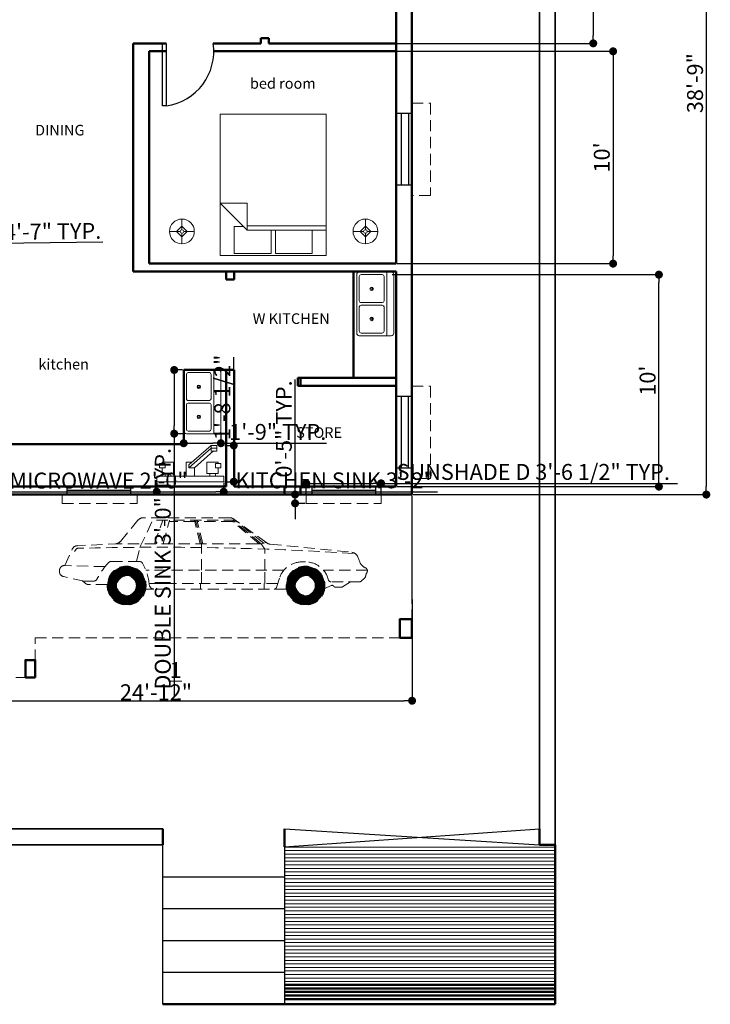
# Model space of a CAD drawing. Units: inches. Extents: x 2050 to 6806, y 2092 to 5743.
# Tile 2 of 8: x 2600 to 2991, y 2149 to 2706. Entities that reach past the tile are written whole.
import ezdxf

# ---------------------------------------------------------------- set-up
doc = ezdxf.new("R2010")
doc.units = ezdxf.units.IN
doc.linetypes.add('HIDDEN', pattern=[9.525, 6.35, -3.175])
for name, color, linetype, lineweight in [('A-ANNO-DIMS', 2, 'Continuous', 18), ('A-AREA-IDEN', 7, 'Continuous', 18), ('A-DOOR', 2, 'Continuous', 25), ('A-FLOR-FIXT', 4, 'Continuous', 18), ('A-FLOR-OVHD', 30, 'HIDDEN', 18), ('A-FLOR-PATT', 8, 'Continuous', 13), ('A-FLOR-STRS', 3, 'Continuous', 25), ('A-FURN', 5, 'Continuous', 18), ('A-GLAZ', 6, 'Continuous', 25), ('A-WALL', 7, 'Continuous', 50), ('C-PROP', 90, 'Continuous', 35)]:
    doc.layers.add(name, color=color, linetype=linetype, lineweight=lineweight)
doc.styles.get("Standard").update_dxf_attribs({"font": 'arial.ttf'})
doc.dimstyles.new('ISO-25', dxfattribs={"dimtxt": 9, "dimasz": 4.5, "dimexe": 1.25, "dimexo": 0.625, "dimtad": 1, "dimdec": 1, "dimlunit": 4, "dimtxsty": 'Standard', "dimblk": 'DOT', "dimcen": 2.5, "dimadec": 0, "dimazin": 0, "dimtfac": 1, "dimtdec": 1, "dimtmove": 0, "dimatfit": 3, "dimldrblk": 'ARCHTICK', "dimfxl": 1, "dimarcsym": 0})

# ---------------------------------------------------------------- blocks, each defined once
blk = doc.blocks.new('Faucet - kit sink front')
for p, q in [((-0.25, 3), (3.75, 6.5)), ((3.75, 6), (-0.25, 2.5)), ((4.1921, 5.5041), (0.75, 2.5)), ((3.75, 6), (3.75, 6.5)), ((3.75, 6.5), (4.75, 6.5)), ((3.75, 5.5), (3.75, 6)), ((4.75, 6), (3.75, 6)), ((4.75, 5.5), (3.75, 5.5)), ((4.75, 6.5), (4.75, 6)), ((4.75, 6), (4.75, 5.5)), ((-0.75, 3.5), (0.3192, 3.5)), ((-0.75, 1), (-0.75, 3.5)), ((-0.25, 2.5), (-0.25, 3)), ((0.75, 2.5), (-0.25, 2.5)), ((0.75, 2.5), (0.75, 1)), ((-4.5, 1), (-4.5, 1.5)), ((-3.5, 1.5), (-3.5, 1)), ((3.5, 1.5), (3.5, 1)), ((4.5, 1), (4.5, 1.5))]:
    blk.add_line(p, q)
for points in [[(-5.5, 2.5), (-5.5, 3.25), (-4.5, 3.25), (-4.5, 2.5)], [(5.5, 2.5), (5.5, 3.25), (4.5, 3.25), (4.5, 2.5)], [(-6, 0), (-6, 1), (6, 1), (6, 0)]]:
    blk.add_lwpolyline(points, close=True)
for points in [[(-5, 3.2513), (-5, 3.5), (-3, 3.5), (-3, 1.5), (-5, 1.5), (-5, 2.5)], [(5, 3.2513), (5, 3.5), (3, 3.5), (3, 1.5), (5, 1.5), (5, 2.5)]]:
    blk.add_lwpolyline(points)
blk = doc.blocks.new('Sink-double - 36 in top')
for p, q in [((-18, -4), (18, -4)), ((-0.75, -18.5), (-0.75, -6.5)), ((0.75, -6.5), (0.75, -18.5))]:
    blk.add_line(p, q)
for points in [[(-16.5, 0), (16.5, 0)], [(-18, -19.5), (-18, -1.5)], [(-15.5, -5.5), (-1.75, -5.5)], [(1.75, -5.5), (15.5, -5.5)], [(18, -1.5), (18, -19.5)], [(-16.5, -18.5), (-16.5, -6.5)], [(16.5, -6.5), (16.5, -18.5)], [(16.5, -21), (-16.5, -21)], [(-1.75, -19.5), (-15.5, -19.5)], [(15.5, -19.5), (1.75, -19.5)]]:
    blk.add_lwpolyline(points)
for centre, radius in [((-8.5, -12.5), 1), ((-8.5, -12.5), 0.5), ((8.5, -12.5), 1), ((8.5, -12.5), 0.5)]:
    blk.add_circle(centre, radius)
for centre, radius, start, end in [((-16.5, -1.5), 1.5, 90, 180), ((16.5, -1.5), 1.5, 0, 90), ((-15.5, -6.5), 1, 90, 180), ((-1.75, -6.5), 1, 0, 90), ((1.75, -6.5), 1, 90, 180), ((15.5, -6.5), 1, 0, 90), ((-16.5, -19.5), 1.5, 180, 270), ((-15.5, -18.5), 1, 180, 270), ((-1.75, -18.5), 1, 270, 0), ((1.75, -18.5), 1, 180, 270), ((15.5, -18.5), 1, 270, 0), ((16.5, -19.5), 1.5, 270, 0)]:
    blk.add_arc(centre, radius, start, end)
blk = doc.blocks.new('Bed - Queen')
for p, q in [((0, -80.00003), (0, 0)), ((0, 0), (59.99999, 0)), ((59.99999, 0), (59.99999, -80.00003)), ((7.99999, -1.2), (28.79998, -1.2)), ((7.99999, -14.4), (7.99999, -1.2)), ((28.79998, -1.2), (28.79998, -14.4)), ((31.19999, -1.2), (51.99999, -1.2)), ((31.19999, -14.4), (31.19999, -1.2)), ((51.99999, -1.2), (51.99999, -16.4)), ((0, -14.4), (44.8, -14.4)), ((59.99999, -29.6), (44.8, -14.4)), ((44.8, -14.4), (44.8, -29.6)), ((51.99999, -16.4), (46.79936, -16.4)), ((44.8, -16.8), (0, -16.8)), ((44.8, -29.6), (59.99999, -29.6)), ((59.99999, -80.00003), (0, -80.00003))]:
    blk.add_line(p, q)
blk = doc.blocks.new('Lamp - Table')
for p, q in [((0, 7), (0, 1)), ((-1, 0), (-7, 0)), ((0, 3), (-3, 0)), ((-3, 0), (0, -3)), ((3, 0), (0, 3)), ((0, -3), (3, 0)), ((1, 0), (7, 0)), ((0, -1), (0, -7))]:
    blk.add_line(p, q)
for radius in [7, 1]:
    blk.add_circle((0, 0), radius)
blk = doc.blocks.new('Car - sedan  side')
for p, q in [((-139.53, 35.99), (-129.64, 47.91)), ((-128.57, 32.64), (-121.22, 48.02)), ((-77.81, 49.34), (-126.58, 49.34)), ((-74.7, 48.02), (-121.22, 48.02)), ((-120.32, 34.67), (-115.67, 48.02)), ((-115.4, 34.67), (-111.74, 48.02)), ((-97.55, 47.3), (-111.94, 47.3)), ((-94.41, 34.67), (-97.73, 48.02)), ((-93.72, 34.67), (-97.04, 48.02)), ((-93.03, 34.67), (-96.34, 48.02)), ((-76.26, 47.3), (-96.16, 47.3)), ((-61.08, 34.66), (-76.26, 47.3)), ((-60.02, 34.65), (-76.07, 48.02)), ((-56.87, 35.13), (-75.48, 48.59)), ((-58.54, 34.93), (-74.99, 48.02)), ((-140.23, 34.67), (-163.88, 33.56)), ((-62.28, 34.67), (-140.23, 34.67)), ((-93.72, 19.62), (-93.72, 34.67)), ((-62.28, 34.67), (-60.02, 34.65)), ((-60.02, 34.65), (-58.54, 34.93)), ((-57.97, 31.61), (-60.02, 34.65)), ((-57.21, 35.38), (-58.54, 34.93)), ((-54.93, 34.4), (-8.75, 29.8)), ((-170.93, 22.32), (-166.81, 31.56)), ((-164.57, 31.6), (-165.48, 30.35)), ((-130.39, 24.63), (-128.57, 32.64)), ((-57.97, 19.62), (-57.97, 31.61)), ((-148.26, 21.7), (-171.11, 22.33)), ((-128.78, 24.63), (-144.79, 24.63)), ((-36.97, 24.38), (-34.94, 24.38)), ((-4.21, 24.18), (-5.42, 27.27)), ((-174, 19.51), (-174, 18.91)), ((-47.2, 19.62), (-125.23, 19.62)), ((-93.72, 12.14), (-93.72, 19.62)), ((-57.97, 12.14), (-57.97, 19.62)), ((0, 19.62), (-24.7, 19.62)), ((-160.12, 13.48), (-171.81, 16.16)), ((-159.22, 12.14), (-161.08, 13.7)), ((-155.01, 13.48), (-160.12, 13.48)), ((-147.03, 11.6), (-157.73, 11.6)), ((-50.67, 12.14), (-123.32, 12.14)), ((-94.21, 9.03), (-94.21, 12.14)), ((-58.39, 9.03), (-58.39, 12.14)), ((-51.4, 9.89), (-49.69, 15.14)), ((-4.23, 13.19), (-20.72, 13.19)), ((-9.5, 13.19), (-14.1, 10.2)), ((-3.22, 13.59), (-1.77, 14.97)), ((-120.62, 9.03), (-125.23, 9.03)), ((-45.76, 9.03), (-120.62, 9.03)), ((-20.36, 11.06), (-24.06, 9.44)), ((-18.83, 10.42), (-19.11, 10.76)), ((-14.68, 10.03), (-18.01, 10.03))]:
    blk.add_line(p, q)
at = {"const_width": 5.49}
for points in [[(-127.8, 11, -1), (-144.3, 11, -1)], [(-26.69, 11, -1), (-43.19, 11, -1)]]:
    blk.add_lwpolyline(points, format="xyb", close=True, dxfattribs=at)
for centre, radius in [((-136.05, 11), 11), ((-34.94, 11), 11), ((-136.05, 11), 5.51), ((-34.94, 11), 5.51)]:
    blk.add_circle(centre, radius)
for centre, radius, start, end in [((-126.58, 45.38), 3.97, 90, 140.3029), ((-77.81, 45.38), 3.97, 54.135, 90), ((-163.72, 30.18), 3.38, 92.6827, 155.9736), ((-142.58, 38.53), 3.97, 272.6827, 320.3029), ((-54.54, 38.35), 3.97, 234.135, 264.3123), ((-163.62, 30.91), 1.17, 91.491, 143.9553), ((-118.51, -1702.12), 1734.79, 86.34698, 91.49105), ((-9.15, 25.82), 4, 21.3107, 84.3123), ((-171.18, 19.51), 2.82, 88.4193, 180), ((-118.09, -2.78), 38.85, 136.3964, 152.9097), ((-144.79, 22.64), 1.98, 90, 136.3964), ((-128.78, 22.64), 1.98, 28.1371, 90), ((-157.14, 7.48), 34.14, 6.5135, 28.1371), ((-36.97, 11), 13.38, 90, 161.9732), ((-34.94, 11), 13.38, 13.5864, 90), ((0.9, 26.18), 5.49, 201.3107, 247.7048), ((-171.18, 18.91), 2.82, 180, 257.0905), ((-3.82, 17.12), 2.96, 313.7173, 352.3839), ((-1.92, 19.3), 1.94, 325.3744, 67.7048), ((2.46, 16.28), 3.37, 145.3744, 172.3839), ((-157.73, 13.93), 2.32, 230.1291, 270), ((-155.01, 16.1), 2.62, 270, 332.9097), ((-120.62, 11.65), 2.62, 186.5135, 270), ((-20.72, 14.43), 1.24, 193.5864, 270), ((-19.93, 10.09), 1.06, 39.301, 113.7159), ((-4.23, 14.65), 1.46, 270, 313.7173), ((-52.58, 10.27), 1.24, 270, 341.9732), ((-18.01, 11.09), 1.06, 219.301, 270), ((-14.68, 11.09), 1.06, 270, 303.047)]:
    blk.add_arc(centre, radius, start, end)
blk = doc.blocks.new('_Dot')
at = {"color": 0, "linetype": 'ByBlock', "lineweight": -2}
blk.add_line((-0.5, 0), (-1, 0), dxfattribs=at)
at = {"color": 0, "linetype": 'ByBlock', "const_width": 0.5}
blk.add_lwpolyline([(-0.25, 0, 1), (0.25, 0, 1)], format="xyb", close=True, dxfattribs=at)
blk = doc.blocks.new('*D32')
at = {"layer": 'A-ANNO-DIMS', "color": 0, "lineweight": -2, "transparency": 16777216}
for p, q in [((2532.41, 2436.47), (2532.47, 2319.32)), ((2821.91, 2436.61), (2821.97, 2319.47)), ((2536.97, 2320.57), (2817.47, 2320.71))]:
    blk.add_line(p, q, dxfattribs=at)
at = {"layer": 'Defpoints', "color": 0, "transparency": 16777216}
for p in [(2821.91, 2437.24), (2532.41, 2437.09), (2821.97, 2320.72)]:
    blk.add_point(p, dxfattribs=at)
at = {"layer": 'A-ANNO-DIMS', "color": 0, "lineweight": -2, "transparency": 16777216, "xscale": 4.5, "yscale": 4.5, "zscale": 4.5}
for p, rotation in [((2532.47, 2320.57), 180.0291193537901), ((2821.97, 2320.72), 0.029119353790171)]:
    blk.add_blockref('_Dot', p, dxfattribs=dict(at, rotation=rotation))
at = {"layer": 'A-ANNO-DIMS', "color": 0, "transparency": 16777216, "insert": (2677.21, 2331.81), "char_height": 9, "attachment_point": 5, "rotation": 0.0291}
blk.add_mtext('24\'-1{\\H1x;\\S1/2;}"', dxfattribs=at)
blk = doc.blocks.new('_ArchTick')
at = {"color": 0, "linetype": 'ByBlock', "const_width": 0.15}
blk.add_lwpolyline([(-0.5, -0.5), (0.5, 0.5)], dxfattribs=at)
blk = doc.blocks.new('*D33')
at = {"layer": 'A-ANNO-DIMS', "color": 0, "lineweight": -2, "transparency": 16777216}
for p, q in [((2810.78, 2561.51), (2962.71, 2561.51)), ((2961.46, 2446.24), (2961.46, 2557.01)), ((2813.53, 2441.74), (2962.71, 2441.74))]:
    blk.add_line(p, q, dxfattribs=at)
at = {"layer": 'Defpoints', "color": 0, "transparency": 16777216}
for p in [(2810.15, 2561.51), (2961.46, 2561.51), (2812.91, 2441.74)]:
    blk.add_point(p, dxfattribs=at)
at = {"layer": 'A-ANNO-DIMS', "color": 0, "lineweight": -2, "transparency": 16777216, "xscale": 4.5, "yscale": 4.5, "zscale": 4.5}
for p, rotation in [((2961.46, 2561.51), 90), ((2961.46, 2441.74), 270)]:
    blk.add_blockref('_Dot', p, dxfattribs=dict(at, rotation=rotation))
at = {"layer": 'A-ANNO-DIMS', "color": 0, "transparency": 16777216, "insert": (2956.24, 2501.62), "char_height": 9, "attachment_point": 5, "rotation": 90}
blk.add_mtext("10'", dxfattribs=at)
blk = doc.blocks.new('*D34')
at = {"layer": 'A-ANNO-DIMS', "color": 0, "lineweight": -2, "transparency": 16777216}
for p, q in [((2822.53, 2902.24), (2989.52, 2902.24)), ((2988.27, 2897.74), (2988.27, 2441.74)), ((2822.53, 2437.24), (2989.52, 2437.24))]:
    blk.add_line(p, q, dxfattribs=at)
at = {"layer": 'Defpoints', "color": 0, "transparency": 16777216}
for p in [(2821.91, 2902.24), (2821.91, 2437.24), (2988.27, 2437.24)]:
    blk.add_point(p, dxfattribs=at)
at = {"layer": 'A-ANNO-DIMS', "color": 0, "lineweight": -2, "transparency": 16777216, "xscale": 4.5, "yscale": 4.5, "zscale": 4.5}
for p, rotation in [((2988.27, 2902.24), 90), ((2988.27, 2437.24), 270)]:
    blk.add_blockref('_Dot', p, dxfattribs=dict(at, rotation=rotation))
at = {"layer": 'A-ANNO-DIMS', "color": 0, "transparency": 16777216, "insert": (2983.05, 2669.74), "char_height": 9, "attachment_point": 5, "rotation": 90}
blk.add_mtext('38\'-9"', dxfattribs=at)
blk = doc.blocks.new('*D35')
at = {"layer": 'A-ANNO-DIMS', "color": 0, "lineweight": -2, "transparency": 16777216}
for p, q in [((2813.53, 2687.74), (2936.83, 2687.74)), ((2935.58, 2683.24), (2935.58, 2572.24)), ((2813.53, 2567.74), (2936.83, 2567.74))]:
    blk.add_line(p, q, dxfattribs=at)
at = {"layer": 'Defpoints', "color": 0, "transparency": 16777216}
for p in [(2812.91, 2687.74), (2812.91, 2567.74), (2935.58, 2567.74)]:
    blk.add_point(p, dxfattribs=at)
at = {"layer": 'A-ANNO-DIMS', "color": 0, "lineweight": -2, "transparency": 16777216, "xscale": 4.5, "yscale": 4.5, "zscale": 4.5}
for p, rotation in [((2935.58, 2687.74), 90), ((2935.58, 2567.74), 270)]:
    blk.add_blockref('_Dot', p, dxfattribs=dict(at, rotation=rotation))
at = {"layer": 'A-ANNO-DIMS', "color": 0, "transparency": 16777216, "insert": (2930.36, 2627.74), "char_height": 9, "attachment_point": 5, "rotation": 90}
blk.add_mtext("10'", dxfattribs=at)
blk = doc.blocks.new('*D36')
at = {"layer": 'A-ANNO-DIMS', "color": 0, "lineweight": -2, "transparency": 16777216}
for p, q in [((2809.63, 2740.24), (2925.62, 2740.24)), ((2924.37, 2735.74), (2924.37, 2696.74)), ((2813.53, 2692.24), (2925.62, 2692.24))]:
    blk.add_line(p, q, dxfattribs=at)
at = {"layer": 'Defpoints', "color": 0, "transparency": 16777216}
for p in [(2809.01, 2740.24), (2812.91, 2692.24), (2924.37, 2692.24)]:
    blk.add_point(p, dxfattribs=at)
at = {"layer": 'A-ANNO-DIMS', "color": 0, "lineweight": -2, "transparency": 16777216, "xscale": 4.5, "yscale": 4.5, "zscale": 4.5}
for p, rotation in [((2924.37, 2740.24), 90), ((2924.37, 2692.24), 270)]:
    blk.add_blockref('_Dot', p, dxfattribs=dict(at, rotation=rotation))
at = {"layer": 'A-ANNO-DIMS', "color": 0, "transparency": 16777216, "insert": (2919.24, 2716.24), "char_height": 9, "attachment_point": 5, "rotation": 90}
blk.add_mtext("4'", dxfattribs=at)
blk = doc.blocks.new('DOOR-750')
blk.add_lwpolyline([(28.97, 0), (26.83, 0), (26.83, 35.38), (28.97, 35.38)], close=True)
blk.add_arc((31.25, 4.42), 31.27, 98.1233, 188.1233)
blk = doc.blocks.new('WIN-1050')
for p, q in [((0, 40.58), (9, 40.58)), ((2.5, 0), (2.5, 40.58)), ((6.5, 0), (6.5, 40.58)), ((0, 0), (9, 0))]:
    blk.add_line(p, q)
blk = doc.blocks.new('SUNSHADE-A')
for p, q in [((0, 52.08), (10.45, 52.08)), ((10.45, 52.08), (10.45, 0)), ((10.45, 0), (0, 0))]:
    blk.add_line(p, q)
blk = doc.blocks.new('SUNSHADE-D')
for p, q in [((0, 4.96), (0, 0)), ((0, 0), (42.28, 0)), ((42.28, 0), (42.28, 4.96))]:
    blk.add_line(p, q)
blk = doc.blocks.new('*D85')
at = {"layer": 'A-ANNO-DIMS', "color": 0, "lineweight": -2, "transparency": 16777216}
for p, q in [((2762.19, 2437.86), (2762.19, 2444.83)), ((2766.69, 2443.58), (2799.97, 2443.58)), ((2804.47, 2437.86), (2804.47, 2444.83)), ((2804.47, 2443.58), (2971.94, 2443.58))]:
    blk.add_line(p, q, dxfattribs=at)
at = {"layer": 'Defpoints', "color": 0, "transparency": 16777216}
for p in [(2804.47, 2443.58), (2762.19, 2437.24), (2804.47, 2437.24)]:
    blk.add_point(p, dxfattribs=at)
at = {"layer": 'A-ANNO-DIMS', "color": 0, "lineweight": -2, "transparency": 16777216, "xscale": 4.5, "yscale": 4.5, "zscale": 4.5, "rotation": 180}
blk.add_blockref('_Dot', (2762.19, 2443.58), dxfattribs=at)
at = {"layer": 'A-ANNO-DIMS', "color": 0, "lineweight": -2, "transparency": 16777216, "xscale": 4.5, "yscale": 4.5, "zscale": 4.5}
blk.add_blockref('_Dot', (2804.47, 2443.58), dxfattribs=at)
at = {"layer": 'A-ANNO-DIMS', "color": 0, "transparency": 16777216, "insert": (2890.45, 2448.86), "char_height": 9, "attachment_point": 5}
blk.add_mtext('SUNSHADE D 3\'-6 1/2" TYP.', dxfattribs=at)
blk = doc.blocks.new('*D86')
at = {"layer": 'A-ANNO-DIMS', "color": 0, "lineweight": -2, "transparency": 16777216}
for p, q in [((2755.85, 2441.74), (2755.85, 2502.35)), ((2761.56, 2437.24), (2754.6, 2437.24)), ((2755.85, 2432.27), (2755.85, 2437.24)), ((2761.56, 2432.27), (2754.6, 2432.27)), ((2755.85, 2427.77), (2755.85, 2423.27))]:
    blk.add_line(p, q, dxfattribs=at)
at = {"layer": 'Defpoints', "color": 0, "transparency": 16777216}
for p in [(2755.85, 2437.24), (2762.19, 2437.24), (2762.19, 2432.27)]:
    blk.add_point(p, dxfattribs=at)
at = {"layer": 'A-ANNO-DIMS', "color": 0, "lineweight": -2, "transparency": 16777216, "xscale": 4.5, "yscale": 4.5, "zscale": 4.5}
for p, rotation in [((2755.85, 2437.24), 270), ((2755.85, 2432.27), 90)]:
    blk.add_blockref('_Dot', p, dxfattribs=dict(at, rotation=rotation))
at = {"layer": 'A-ANNO-DIMS', "color": 0, "transparency": 16777216, "insert": (2750.63, 2474.29), "char_height": 9, "attachment_point": 5, "rotation": 90}
blk.add_mtext('0\'-5" TYP.', dxfattribs=at)
blk = doc.blocks.new('*D91')
at = {"layer": 'A-ANNO-DIMS', "color": 0, "lineweight": -2, "transparency": 16777216}
for p, q in [((2692.28, 2507.65), (2686.26, 2507.65)), ((2687.51, 2503.15), (2687.51, 2476.15)), ((2692.28, 2471.65), (2686.26, 2471.65)), ((2687.51, 2471.65), (2687.51, 2323.46))]:
    blk.add_line(p, q, dxfattribs=at)
at = {"layer": 'Defpoints', "color": 0, "transparency": 16777216}
for p in [(2692.91, 2507.65), (2687.51, 2471.65), (2692.91, 2471.65)]:
    blk.add_point(p, dxfattribs=at)
at = {"layer": 'A-ANNO-DIMS', "color": 0, "lineweight": -2, "transparency": 16777216, "xscale": 4.5, "yscale": 4.5, "zscale": 4.5}
for p, rotation in [((2687.51, 2507.65), 90), ((2687.51, 2471.65), 270)]:
    blk.add_blockref('_Dot', p, dxfattribs=dict(at, rotation=rotation))
at = {"layer": 'A-ANNO-DIMS', "color": 0, "transparency": 16777216, "insert": (2682.22, 2395.31), "char_height": 9, "attachment_point": 5, "rotation": 90}
blk.add_mtext('DOUBLE SINK 3\'-0" TYP.', dxfattribs=at)
blk = doc.blocks.new('*D92')
at = {"layer": 'A-ANNO-DIMS', "color": 0, "lineweight": -2, "transparency": 16777216}
for p, q in [((2692.91, 2471.03), (2692.91, 2465)), ((2713.91, 2471.03), (2713.91, 2465)), ((2697.41, 2466.25), (2709.41, 2466.25)), ((2713.91, 2466.25), (2773.67, 2466.25))]:
    blk.add_line(p, q, dxfattribs=at)
at = {"layer": 'Defpoints', "color": 0, "transparency": 16777216}
for p in [(2692.91, 2471.65), (2713.91, 2471.65), (2713.91, 2466.25)]:
    blk.add_point(p, dxfattribs=at)
at = {"layer": 'A-ANNO-DIMS', "color": 0, "lineweight": -2, "transparency": 16777216, "xscale": 4.5, "yscale": 4.5, "zscale": 4.5, "rotation": 180}
blk.add_blockref('_Dot', (2692.91, 2466.25), dxfattribs=at)
at = {"layer": 'A-ANNO-DIMS', "color": 0, "lineweight": -2, "transparency": 16777216, "xscale": 4.5, "yscale": 4.5, "zscale": 4.5}
blk.add_blockref('_Dot', (2713.91, 2466.25), dxfattribs=at)
at = {"layer": 'A-ANNO-DIMS', "color": 0, "transparency": 16777216, "insert": (2746.04, 2471.47), "char_height": 9, "attachment_point": 5}
blk.add_mtext('1\'-9" TYP.', dxfattribs=at)
blk = doc.blocks.new('*D94')
at = {"layer": 'A-ANNO-DIMS', "color": 0, "lineweight": -2, "transparency": 16777216}
for p, q in [((2530.99, 2591.58), (2531.18, 2577.3)), ((2585.99, 2592.28), (2586.17, 2578.01)), ((2535.66, 2578.61), (2581.66, 2579.2)), ((2586.16, 2579.26), (2647.12, 2580.04))]:
    blk.add_line(p, q, dxfattribs=at)
at = {"layer": 'Defpoints', "color": 0, "transparency": 16777216}
for p in [(2530.98, 2592.2), (2585.98, 2592.91), (2586.16, 2579.26)]:
    blk.add_point(p, dxfattribs=at)
at = {"layer": 'A-ANNO-DIMS', "color": 0, "lineweight": -2, "transparency": 16777216, "xscale": 4.5, "yscale": 4.5, "zscale": 4.5}
for p, rotation in [((2531.16, 2578.55), 180.7337264995931), ((2586.16, 2579.26), 0.7337264995931003)]:
    blk.add_blockref('_Dot', p, dxfattribs=dict(at, rotation=rotation))
at = {"layer": 'A-ANNO-DIMS', "color": 0, "transparency": 16777216, "insert": (2618.82, 2584.8), "char_height": 9, "attachment_point": 5, "rotation": 0.7337}
blk.add_mtext('4\'-7" TYP.', dxfattribs=at)
blk = doc.blocks.new('*D105')
at = {"layer": 'A-ANNO-DIMS', "color": 0, "lineweight": -2, "transparency": 16777216}
for p, q in [((2562.63, 2441.66), (2562.63, 2437.44)), ((2567.13, 2438.69), (2582.13, 2438.69)), ((2586.63, 2441.66), (2586.63, 2437.44)), ((2586.63, 2438.69), (2698.32, 2438.69))]:
    blk.add_line(p, q, dxfattribs=at)
at = {"layer": 'Defpoints', "color": 0, "transparency": 16777216}
for p in [(2562.63, 2442.29), (2586.63, 2442.29), (2586.63, 2438.69)]:
    blk.add_point(p, dxfattribs=at)
at = {"layer": 'A-ANNO-DIMS', "color": 0, "lineweight": -2, "transparency": 16777216, "xscale": 4.5, "yscale": 4.5, "zscale": 4.5, "rotation": 180}
blk.add_blockref('_Dot', (2562.63, 2438.69), dxfattribs=at)
at = {"layer": 'A-ANNO-DIMS', "color": 0, "lineweight": -2, "transparency": 16777216, "xscale": 4.5, "yscale": 4.5, "zscale": 4.5}
blk.add_blockref('_Dot', (2586.63, 2438.69), dxfattribs=at)
at = {"layer": 'A-ANNO-DIMS', "color": 0, "transparency": 16777216, "insert": (2644.72, 2443.97), "char_height": 9, "attachment_point": 5}
blk.add_mtext('MICROWAVE 2\'-0"', dxfattribs=at)
blk = doc.blocks.new('*D111')
at = {"layer": 'A-ANNO-DIMS', "color": 0, "lineweight": -2, "transparency": 16777216}
for p, q in [((2677.64, 2443.87), (2677.64, 2437.57)), ((2715.5, 2443.87), (2715.5, 2437.57)), ((2682.14, 2438.82), (2711, 2438.82)), ((2715.5, 2438.82), (2836.29, 2438.82))]:
    blk.add_line(p, q, dxfattribs=at)
at = {"layer": 'Defpoints', "color": 0, "transparency": 16777216}
for p in [(2677.64, 2444.5), (2715.5, 2444.5), (2715.5, 2438.82)]:
    blk.add_point(p, dxfattribs=at)
at = {"layer": 'A-ANNO-DIMS', "color": 0, "lineweight": -2, "transparency": 16777216, "xscale": 4.5, "yscale": 4.5, "zscale": 4.5, "rotation": 180}
blk.add_blockref('_Dot', (2677.64, 2438.82), dxfattribs=at)
at = {"layer": 'A-ANNO-DIMS', "color": 0, "lineweight": -2, "transparency": 16777216, "xscale": 4.5, "yscale": 4.5, "zscale": 4.5}
blk.add_blockref('_Dot', (2715.5, 2438.82), dxfattribs=at)
at = {"layer": 'A-ANNO-DIMS', "color": 0, "transparency": 16777216, "insert": (2778.15, 2444.1), "char_height": 9, "attachment_point": 5}
blk.add_mtext('KITCHEN SINK 3\'-2"', dxfattribs=at)
blk = doc.blocks.new('*D112')
at = {"layer": 'A-ANNO-DIMS', "color": 0, "lineweight": -2, "transparency": 16777216}
for p, q in [((2721.18, 2465), (2721.18, 2514.8)), ((2716.13, 2465), (2722.43, 2465)), ((2721.18, 2449), (2721.18, 2460.5)), ((2716.13, 2444.5), (2722.43, 2444.5))]:
    blk.add_line(p, q, dxfattribs=at)
at = {"layer": 'Defpoints', "color": 0, "transparency": 16777216}
for p in [(2715.5, 2465), (2721.18, 2465), (2715.5, 2444.5)]:
    blk.add_point(p, dxfattribs=at)
at = {"layer": 'A-ANNO-DIMS', "color": 0, "lineweight": -2, "transparency": 16777216, "xscale": 4.5, "yscale": 4.5, "zscale": 4.5}
for p, rotation in [((2721.18, 2465), 90), ((2721.18, 2444.5), 270)]:
    blk.add_blockref('_Dot', p, dxfattribs=dict(at, rotation=rotation))
at = {"layer": 'A-ANNO-DIMS', "color": 0, "transparency": 16777216, "insert": (2715.9, 2492.15), "char_height": 9, "attachment_point": 5, "rotation": 90}
blk.add_mtext('1\'-8 1/2"', dxfattribs=at)

msp = doc.modelspace()

# ---------------------------------------------------------------- hatches: boundary and pattern name
at = {"layer": 'A-FLOR-PATT'}
h = msp.add_hatch(dxfattribs=at)
h.set_pattern_fill('ANSI31', color=256, scale=0.629921, angle=-45, style=0)
h.paths.add_polyline_path([(2749.91, 2224.16), (2902.91, 2224.16), (2902.91, 2238.16), (2749.91, 2238.16)])
h = msp.add_hatch(dxfattribs=at)
h.set_pattern_fill('ANSI31', color=256, scale=0.629921, angle=-45, style=0)
h.paths.add_polyline_path([(2749.91, 2176.16), (2902.91, 2176.16), (2902.91, 2224.16), (2749.91, 2224.16)])
h = msp.add_hatch(dxfattribs=at)
h.set_pattern_fill('ANSI31', color=256, scale=0.629921, angle=-45, style=0)
h.paths.add_polyline_path([(2749.91, 2160.16), (2902.91, 2160.16), (2902.91, 2176.16), (2749.91, 2176.16)])

# ---------------------------------------------------------------- linework, layer by layer
at = {"layer": 'A-DOOR'}
for p, q in [((2749.91, 2248.24), (2893.91, 2239.24)), ((2749.91, 2238.16), (2893.91, 2248.24))]:
    msp.add_line(p, q, dxfattribs=at)
at = {"layer": 'A-FLOR-OVHD'}
for p, q in [((2821.91, 2356.35), (2821.91, 2437.24)), ((2608.94, 2333.88), (2608.94, 2356.35)), ((2608.94, 2356.35), (2821.91, 2356.35)), ((2359.91, 2333.88), (2608.94, 2333.88))]:
    msp.add_line(p, q, dxfattribs=at)
at = {"layer": 'A-FLOR-STRS'}
for p, q in [((2681.02, 2149.16), (2681.02, 2239.24)), ((2749.91, 2238.16), (2749.91, 2149.24))]:
    msp.add_line(p, q, dxfattribs=at)
for points in [[(2681.02, 2221.24), (2749.91, 2221.24)], [(2681.02, 2203.24), (2749.91, 2203.24)], [(2681.02, 2185.24), (2749.91, 2185.24)], [(2681.02, 2167.24), (2749.91, 2167.24)], [(2681.02, 2149.24), (2749.91, 2149.24)]]:
    msp.add_lwpolyline(points, dxfattribs=at)
at = {"layer": 'A-GLAZ'}
for p, q in [((2626.91, 2441.74), (2626.91, 2437.24)), ((2626.91, 2439.74), (2645.82, 2439.74)), ((2626.91, 2439.74), (2662.91, 2439.74)), ((2662.91, 2441.74), (2662.91, 2437.24)), ((2765.24, 2441.66), (2765.24, 2437.16)), ((2765.24, 2439.66), (2801.24, 2439.66)), ((2765.24, 2439.66), (2784.16, 2439.66)), ((2801.24, 2441.66), (2801.24, 2437.16))]:
    msp.add_line(p, q, dxfattribs=at)
at = {"layer": 'A-WALL'}
for p, q in [((2821.91, 2437.24), (2821.91, 2902.24)), ((2812.91, 2567.74), (2812.91, 2740.24)), ((2736.41, 2692.24), (2736.41, 2695.24)), ((2736.41, 2695.24), (2740.91, 2695.24)), ((2740.91, 2692.24), (2740.91, 2695.24)), ((2664.41, 2692.24), (2664.41, 2563.24)), ((2683.05, 2692.24), (2664.41, 2692.24)), ((2673.41, 2687.74), (2673.41, 2567.74)), ((2683.05, 2687.74), (2673.41, 2687.74)), ((2736.41, 2692.24), (2709.59, 2692.24)), ((2736.41, 2687.74), (2709.9, 2687.74)), ((2736.41, 2692.24), (2721.41, 2692.24)), ((2812.91, 2687.74), (2736.41, 2687.74)), ((2812.91, 2692.24), (2740.91, 2692.24)), ((2812.91, 2567.74), (2673.41, 2567.74)), ((2812.91, 2567.74), (2736.41, 2567.74)), ((2721.41, 2563.24), (2664.41, 2563.24)), ((2716.91, 2558.74), (2716.91, 2563.24)), ((2812.91, 2563.24), (2721.41, 2563.24)), ((2721.41, 2558.74), (2721.41, 2563.24)), ((2788.91, 2503.24), (2788.91, 2563.24)), ((2812.91, 2441.74), (2812.91, 2563.24)), ((2721.41, 2558.74), (2716.91, 2558.74)), ((2692.91, 2465.74), (2692.91, 2507.74)), ((2692.91, 2507.74), (2716.91, 2507.74)), ((2716.91, 2441.74), (2716.91, 2507.74)), ((2721.41, 2507.74), (2716.91, 2507.74)), ((2721.41, 2441.74), (2721.41, 2507.74)), ((2721.41, 2441.74), (2721.41, 2498.74)), ((2812.91, 2503.24), (2757.41, 2503.24)), ((2757.41, 2498.74), (2757.41, 2503.24)), ((2812.91, 2498.74), (2757.41, 2498.74)), ((2560.91, 2465.74), (2692.91, 2465.74)), ((2536.91, 2441.74), (2716.91, 2441.74)), ((2536.91, 2437.24), (2821.91, 2437.24)), ((2626.91, 2441.74), (2645.82, 2441.74)), ((2721.41, 2441.74), (2812.91, 2441.74)), ((2749.91, 2437.24), (2749.91, 2441.74)), ((2681.03, 2248.24), (2681.02, 2239.24)), ((2749.91, 2238.16), (2749.91, 2248.24)), ((2893.91, 2239.24), (2893.91, 2248.24)), ((2902.91, 2239.24), (2893.91, 2239.24)), ((2902.91, 2239.24), (2897.91, 2239.05)), ((2902.91, 2239.24), (2902.91, 2149.16)), ((2902.91, 2160.16), (2749.91, 2160.16)), ((2902.91, 2158.16), (2749.91, 2158.16)), ((2902.91, 2156.16), (2749.91, 2156.16)), ((2902.91, 2154.16), (2749.91, 2154.16)), ((2902.91, 2149.16), (2681.02, 2149.16)), ((2902.91, 2152.16), (2749.91, 2152.16))]:
    msp.add_line(p, q, dxfattribs=at)
for points in [[(2758.91, 2498.74), (2758.91, 2503.24)], [(2758.91, 2498.74), (2758.91, 2503.24)], [(2758.91, 2437.24), (2758.91, 2441.74)], [(2758.91, 2437.24), (2758.91, 2441.74)]]:
    msp.add_lwpolyline(points, dxfattribs=at)
for points in [[(2821.91, 2356.35), (2814.96, 2356.35), (2814.96, 2366.74), (2821.91, 2366.74)], [(2608.94, 2333.88), (2603.46, 2333.88), (2603.46, 2343.66), (2608.94, 2343.66)]]:
    msp.add_lwpolyline(points, close=True, dxfattribs=at)
at = {"layer": 'C-PROP'}
for p, q in [((2893.91, 2248.24), (2893.91, 2950.24)), ((2311.91, 2248.24), (2681.03, 2248.24))]:
    msp.add_line(p, q, dxfattribs=at)
msp.add_lwpolyline([(2902.91, 2239.24), (2902.91, 2959.24), (2302.91, 2959.24), (2302.91, 2239.24), (2681.02, 2239.24)], dxfattribs=at)

# ---------------------------------------------------------------- block references
at = {"layer": 'A-DOOR', "rotation": 180}
msp.add_blockref('DOOR-750', (2709.88, 2692.24), dxfattribs=at)
at = {"layer": 'A-FLOR-FIXT', "rotation": 270}
for p in [(2811.65, 2545.01), (2713.91, 2489.65)]:
    msp.add_blockref('Sink-double - 36 in top', p, dxfattribs=at)
at = {"layer": 'A-FLOR-FIXT', "xscale": 3.154993944848655, "yscale": 3.154993944848655, "zscale": 3.154993944848655}
msp.add_blockref('Faucet - kit sink front', (2696.57, 2444.5), dxfattribs=at)
at = {"layer": 'A-FLOR-OVHD'}
for name, p in [('SUNSHADE-A', (2821.91, 2606.31)), ('SUNSHADE-A', (2821.91, 2446.34)), ('SUNSHADE-D', (2624.28, 2432.27)), ('SUNSHADE-D', (2762.19, 2432.27)), ('Car - sedan  side', (2796.68, 2374.8))]:
    msp.add_blockref(name, p, dxfattribs=at)
at = {"layer": 'A-FURN', "rotation": 180}
msp.add_blockref('Bed - Queen', (2773.48, 2572.29), dxfattribs=at)
at = {"layer": 'A-FURN'}
for p in [(2691.88, 2585.93), (2795.6, 2585.93)]:
    msp.add_blockref('Lamp - Table', p, dxfattribs=at)
at = {"layer": 'A-GLAZ', "rotation": 180}
for p in [(2822.38, 2652.6), (2822.21, 2492.65)]:
    msp.add_blockref('WIN-1050', p, dxfattribs=at)

# ---------------------------------------------------------------- texts
at = {"layer": 'A-AREA-IDEN'}
for s, p in [('bed room', (2730.32, 2666.58)), ('DINING', (2608.9, 2640.18)), ('W KITCHEN', (2731.89, 2533.66)), ('kitchen', (2610.78, 2507.91)), ('STORE', (2756.47, 2469.28))]:
    msp.add_text(s, height=6, dxfattribs=at).set_placement(p)

# ---------------------------------------------------------------- dimensions: what is measured, and where the dimension line sits
at = {"layer": 'A-ANNO-DIMS'}
for base, p1, p2, override, picture, middle in [((2988.27, 2437.24), (2821.91, 2902.24), (2821.91, 2437.24), {"dimclrd": 0, "dimclre": 0, "dimclrt": 0}, '*D34', (2983.05, 2669.74)), ((2924.37, 2692.24), (2809.01, 2740.24), (2812.91, 2692.24), {"dimclrd": 0, "dimclre": 0, "dimclrt": 0}, '*D36', (2919.24, 2716.24)), ((2935.58, 2567.74), (2812.91, 2687.74), (2812.91, 2567.74), {"dimclrd": 0, "dimclre": 0, "dimclrt": 0}, '*D35', (2930.36, 2627.74)), ((2961.46, 2561.51), (2812.91, 2441.74), (2810.15, 2561.51), {"dimclrd": 0, "dimclre": 0, "dimclrt": 0}, '*D33', (2956.24, 2501.62)), ((2721.18, 2465), (2715.5, 2444.5), (2715.5, 2465), {"dimdec": 1, "dimlfac": 1, "dimrnd": 0, "dimzin": 1, "dimdsep": 46, "dimlunit": 4, "dimfrac": 2}, '*D112', (2715.9, 2492.15))]:
    dim = msp.add_linear_dim(base=base, p1=p1, p2=p2, angle=90, dimstyle='ISO-25', override=override, dxfattribs=at)
    dim.commit()
    dim.dimension.update_dxf_attribs({"geometry": picture, "text_midpoint": middle})
for base, p1, p2, angle, text, picture, middle in [((2586.16, 2579.26), (2530.98, 2592.2), (2585.98, 2592.91), 0.7337, '<> TYP.', '*D94', (2618.82, 2584.8)), ((2687.51, 2471.65), (2692.91, 2507.65), (2692.91, 2471.65), 270, 'DOUBLE SINK <> TYP.', '*D91', (2682.22, 2395.31)), ((2755.85, 2437.24), (2762.19, 2432.27), (2762.19, 2437.24), 90, '<> TYP.', '*D86', (2750.63, 2474.29))]:
    dim = msp.add_linear_dim(base=base, p1=p1, p2=p2, angle=angle, text=text, dimstyle='ISO-25', override={"dimdec": 1, "dimlfac": 1, "dimrnd": 0, "dimzin": 1, "dimdsep": 46, "dimlunit": 4, "dimfrac": 2}, dxfattribs=at)
    dim.commit()
    dim.dimension.update_dxf_attribs({"geometry": picture, "text_midpoint": middle})
for base, p1, p2, text, picture, middle in [((2713.91, 2466.25), (2692.91, 2471.65), (2713.91, 2471.65), '<> TYP.', '*D92', (2746.04, 2471.47)), ((2804.47, 2443.58), (2762.19, 2437.24), (2804.47, 2437.24), 'SUNSHADE D <> TYP.', '*D85', (2890.45, 2448.86)), ((2715.5, 2438.82), (2677.64, 2444.5), (2715.5, 2444.5), 'KITCHEN SINK <>', '*D111', (2778.15, 2444.1)), ((2586.63, 2438.69), (2562.63, 2442.29), (2586.63, 2442.29), 'MICROWAVE <>', '*D105', (2644.72, 2443.97))]:
    dim = msp.add_linear_dim(base=base, p1=p1, p2=p2, text=text, dimstyle='ISO-25', override={"dimdec": 1, "dimlfac": 1, "dimrnd": 0, "dimzin": 1, "dimdsep": 46, "dimlunit": 4, "dimfrac": 2}, dxfattribs=at)
    dim.commit()
    dim.dimension.update_dxf_attribs({"geometry": picture, "text_midpoint": middle})
dim = msp.add_aligned_dim(p1=(2532.41, 2437.09), p2=(2821.91, 2437.24), distance=-116.52, dimstyle='ISO-25', override={"dimclrd": 0, "dimclre": 0, "dimclrt": 0}, dxfattribs=at)
dim.commit()
dim.dimension.update_dxf_attribs({"geometry": '*D32', "text_midpoint": (2677.21, 2331.81)})

doc.saveas('drawing.dxf')
